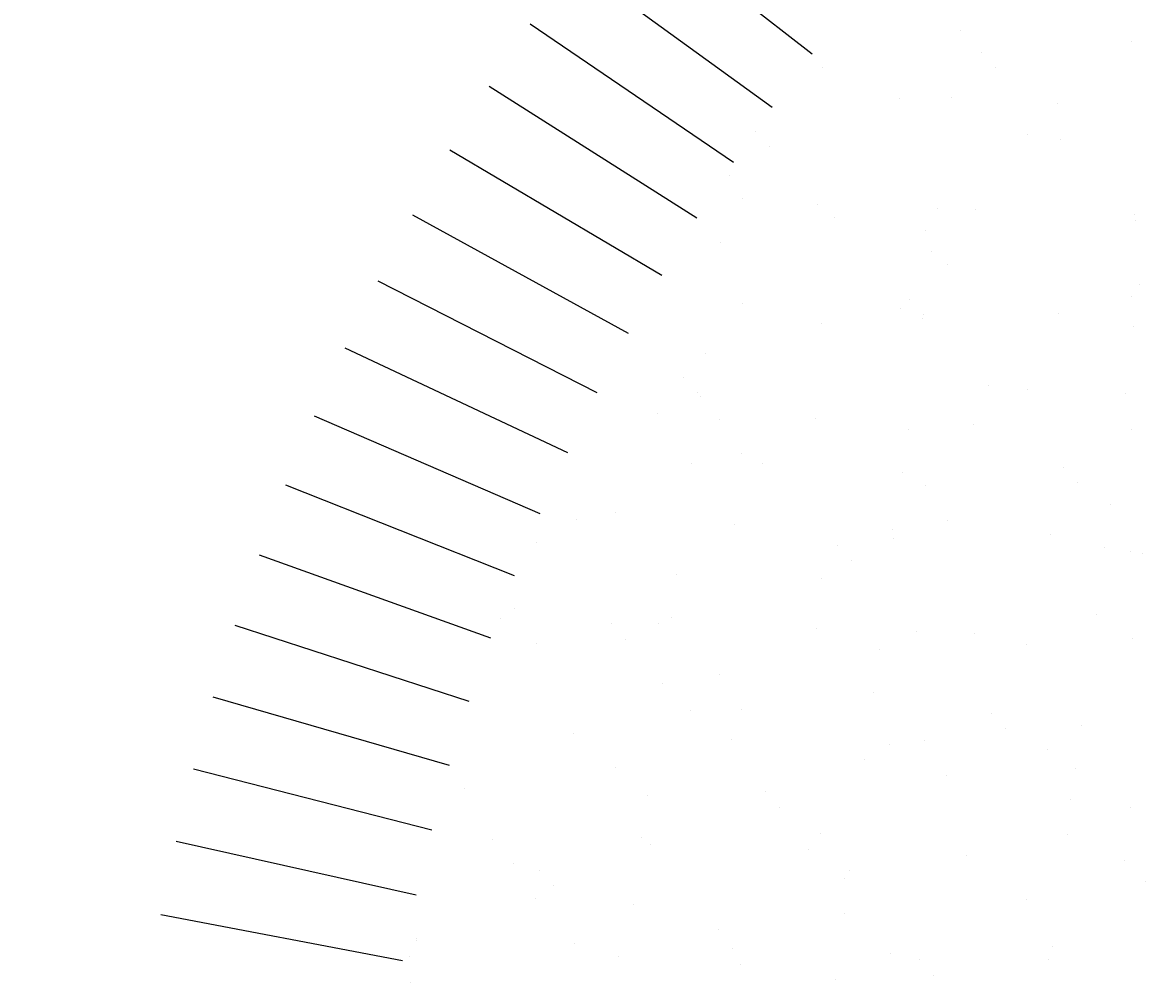
# Model space of a CAD drawing. Units: millimetres. Extents: x -857 to 54106, y -13666 to 13947.
# Tile 35 of 41: x 30856 to 31475, y 9986 to 10517. Entities that reach past the tile are written whole.
import ezdxf

# ---------------------------------------------------------------- set-up
doc = ezdxf.new("R2010")
doc.units = ezdxf.units.MM
doc.layers.add('A-ANNO-DIMS', color=2, linetype='Continuous', lineweight=18)
doc.layers.add('A-FURN', color=21, linetype='Continuous', lineweight=18)
doc.layers.add('A-HT', color=15, linetype='Continuous')
doc.styles.get("Standard").update_dxf_attribs({"font": 'arial.ttf'})
doc.dimstyles.new('ISO-25', dxfattribs={"dimtxt": 2.5, "dimasz": 2.5, "dimexe": 1.25, "dimexo": 0.625, "dimtad": 1, "dimtxsty": 'Standard', "dimcen": 2.5, "dimadec": 0, "dimazin": 0, "dimtfac": 1, "dimtmove": 0, "dimatfit": 3, "dimfxl": 1, "dimarcsym": 0})

# ---------------------------------------------------------------- blocks, each defined once
blk = doc.blocks.new('*X18')
at = {"color": 0}
for p, q in [((1.75374, 2.82274), (1.75374, 2.82274)), ((1.76978, 2.82215), (1.76978, 2.82215)), ((1.74276, 2.81864), (1.74276, 2.81864)), ((1.74375, 2.81872), (1.74375, 2.81872)), ((1.65142, 2.78914), (1.65142, 2.78914)), ((1.54742, 2.7675), (1.54742, 2.7675)), ((1.68246, 2.77237), (1.68246, 2.77237)), ((1.69713, 2.75932), (1.69713, 2.75932)), ((1.54142, 2.75904), (1.54142, 2.75904)), ((1.56251, 2.74561), (1.56251, 2.74561)), ((1.71821, 2.74589), (1.71821, 2.74589)), ((1.50111, 2.74526), (1.50111, 2.74526)), ((1.70118, 2.74354), (1.70118, 2.74354)), ((1.7104, 2.73509), (1.7104, 2.73509)), ((1.48712, 2.72124), (1.48712, 2.72124)), ((1.618, 2.72291), (1.618, 2.72291)), ((1.74591, 2.72229), (1.74591, 2.72229)), ((1.55088, 2.69965), (1.55088, 2.69965)), ((1.48271, 2.69697), (1.48271, 2.69697)), ((1.56009, 2.69121), (1.56009, 2.69121)), ((1.63841, 2.69725), (1.63841, 2.69725)), ((1.7539, 2.69523), (1.7539, 2.69523)), ((1.72194, 2.68639), (1.72194, 2.68639)), ((1.65526, 2.67761), (1.65526, 2.67761)), ((1.68129, 2.68104), (1.68129, 2.68104)), ((1.42266, 2.67178), (1.42266, 2.67178)), ((1.55057, 2.67116), (1.55057, 2.67116)), ((1.68561, 2.67603), (1.68561, 2.67603)), ((1.58735, 2.66867), (1.58735, 2.66867)), ((1.52067, 2.65989), (1.52067, 2.65989)), ((1.5467, 2.66332), (1.5467, 2.66332)), ((1.40057, 2.65577), (1.40057, 2.65577)), ((1.45276, 2.65095), (1.45276, 2.65095)), ((1.60359, 2.65135), (1.60359, 2.65135)), ((1.40979, 2.64732), (1.40979, 2.64732)), ((1.41211, 2.6456), (1.41211, 2.6456)), ((1.38609, 2.64217), (1.38609, 2.64217)), ((1.31817, 2.63323), (1.31817, 2.63323)), ((1.4261, 2.63355), (1.4261, 2.63355)), ((1.5818, 2.63383), (1.5818, 2.63383)), ((1.73751, 2.63412), (1.73751, 2.63412)), ((1.27752, 2.62788), (1.27752, 2.62788)), ((1.49027, 2.6249), (1.49027, 2.6249)), ((1.62115, 2.62657), (1.62115, 2.62657)), ((1.74906, 2.62595), (1.74906, 2.62595)), ((1.29147, 2.61984), (1.29147, 2.61984)), ((1.35523, 2.62003), (1.35523, 2.62003)), ((1.44718, 2.62012), (1.44718, 2.62012)), ((1.60289, 2.6204), (1.60289, 2.6204)), ((1.7586, 2.62069), (1.7586, 2.62069)), ((1.25027, 2.61189), (1.25027, 2.61189)), ((1.25948, 2.60344), (1.25948, 2.60344)), ((1.45329, 2.60747), (1.45329, 2.60747)), ((1.65336, 2.60575), (1.65336, 2.60575)), ((1.66258, 2.5973), (1.66258, 2.5973)), ((1.42581, 2.57544), (1.42581, 2.57544)), ((1.55372, 2.57482), (1.55372, 2.57482)), ((1.68876, 2.57969), (1.68876, 2.57969)), ((1.21167, 2.5712), (1.21167, 2.5712)), ((1.29493, 2.57377), (1.29493, 2.57377)), ((1.36738, 2.57148), (1.36738, 2.57148)), ((1.52309, 2.57176), (1.52309, 2.57176)), ((1.67879, 2.57205), (1.67879, 2.57205)), ((1.30298, 2.56358), (1.30298, 2.56358)), ((1.50305, 2.56186), (1.50305, 2.56186)), ((1.76804, 2.563), (1.76804, 2.563)), ((1.70136, 2.55422), (1.70136, 2.55422)), ((1.70607, 2.55744), (1.70607, 2.55744)), ((1.72739, 2.55765), (1.72739, 2.55765)), ((1.51227, 2.55342), (1.51227, 2.55342)), ((1.63345, 2.54528), (1.63345, 2.54528)), ((1.56677, 2.53651), (1.56677, 2.53651)), ((1.5928, 2.53993), (1.5928, 2.53993)), ((1.49342, 2.52856), (1.49342, 2.52856)), ((1.49886, 2.52756), (1.49886, 2.52756)), ((1.6243, 2.53023), (1.6243, 2.53023)), ((1.75221, 2.52961), (1.75221, 2.52961)), ((1.23047, 2.5243), (1.23047, 2.5243)), ((1.35838, 2.52369), (1.35838, 2.52369)), ((1.45821, 2.52221), (1.45821, 2.52221)), ((1.35275, 2.51798), (1.35275, 2.51798)), ((1.43218, 2.51879), (1.43218, 2.51879)), ((1.55577, 2.51356), (1.55577, 2.51356)), ((1.31077, 2.50806), (1.31077, 2.50806)), ((1.36196, 2.50953), (1.36196, 2.50953)), ((1.36427, 2.50985), (1.36427, 2.50985)), ((1.46648, 2.50835), (1.46648, 2.50835)), ((1.62219, 2.50863), (1.62219, 2.50863)), ((1.75584, 2.51184), (1.75584, 2.51184)), ((1.2976, 2.50107), (1.2976, 2.50107)), ((1.32362, 2.50449), (1.32362, 2.50449)), ((1.76506, 2.50339), (1.76506, 2.50339)), ((1.33186, 2.49463), (1.33186, 2.49463)), ((1.48756, 2.49491), (1.48756, 2.49491)), ((1.64327, 2.4952), (1.64327, 2.4952)), ((1.18903, 2.48677), (1.18903, 2.48677)), ((1.22968, 2.49213), (1.22968, 2.49213)), ((1.42896, 2.47909), (1.42896, 2.47909)), ((1.69191, 2.48335), (1.69191, 2.48335)), ((1.20244, 2.4741), (1.20244, 2.4741)), ((1.29808, 2.47743), (1.29808, 2.47743)), ((1.55687, 2.47848), (1.55687, 2.47848)), ((1.21166, 2.46565), (1.21166, 2.46565)), ((1.40546, 2.46967), (1.40546, 2.46967)), ((1.60553, 2.46796), (1.60553, 2.46796)), ((1.61475, 2.45951), (1.61475, 2.45951)), ((1.25205, 2.44599), (1.25205, 2.44599)), ((1.40776, 2.44627), (1.40776, 2.44627)), ((1.56347, 2.44656), (1.56347, 2.44656)), ((1.71918, 2.44684), (1.71918, 2.44684)), ((1.49657, 2.43222), (1.49657, 2.43222)), ((1.62745, 2.43388), (1.62745, 2.43388)), ((1.74746, 2.43084), (1.74746, 2.43084)), ((1.75536, 2.43327), (1.75536, 2.43327)), ((1.23362, 2.42796), (1.23362, 2.42796)), ((1.25516, 2.42579), (1.25516, 2.42579)), ((1.36153, 2.42735), (1.36153, 2.42735)), ((1.45523, 2.42407), (1.45523, 2.42407)), ((1.65825, 2.41965), (1.65825, 2.41965)), ((1.67955, 2.42189), (1.67955, 2.42189)), ((1.46444, 2.41563), (1.46444, 2.41563)), ((1.61287, 2.41312), (1.61287, 2.41312)), ((1.6389, 2.41654), (1.6389, 2.41654)), ((1.54496, 2.40418), (1.54496, 2.40418)), ((1.50431, 2.39882), (1.50431, 2.39882)), ((1.47828, 2.3954), (1.47828, 2.3954)), ((1.35115, 2.38286), (1.35115, 2.38286)), ((1.41037, 2.38646), (1.41037, 2.38646)), ((1.43211, 2.38275), (1.43211, 2.38275)), ((1.50686, 2.38314), (1.50686, 2.38314)), ((1.66257, 2.38342), (1.66257, 2.38342)), ((1.69506, 2.38701), (1.69506, 2.38701)), ((1.19545, 2.38258), (1.19545, 2.38258)), ((1.30123, 2.38108), (1.30123, 2.38108)), ((1.30492, 2.38019), (1.30492, 2.38019)), ((1.3437, 2.37768), (1.3437, 2.37768)), ((1.36972, 2.38111), (1.36972, 2.38111)), ((1.56002, 2.38214), (1.56002, 2.38214)), ((1.50794, 2.37577), (1.50794, 2.37577)), ((1.70802, 2.37405), (1.70802, 2.37405))]:
    blk.add_line(p, q, dxfattribs=at)
blk = doc.blocks.new('A$C6796526C')
at = {"layer": 'A-HT'}
for p, q in [((0.65322, 0.4228), (0.56128, 0.30428)), ((0.68588, 0.39828), (0.59771, 0.27693)), ((0.71929, 0.3748), (0.63498, 0.25073)), ((0.75343, 0.35237), (0.67305, 0.22572)), ((0.78825, 0.33104), (0.71189, 0.20192)), ((0.82372, 0.3108), (0.75146, 0.17936)), ((0.85981, 0.29169), (0.79171, 0.15804)), ((0.89649, 0.27372), (0.83262, 0.138)), ((0.93371, 0.25692), (0.87414, 0.11926)), ((0.97144, 0.24129), (0.91622, 0.10182)), ((1.00964, 0.22686), (0.95883, 0.08572)), ((1.04828, 0.21363), (1.00193, 0.07097)), ((1.08731, 0.20162), (1.04546, 0.05757)), ((1.1267, 0.19084), (1.0894, 0.04555)), ((1.16641, 0.18131), (1.13369, 0.03492)), ((1.2064, 0.17303), (1.1783, 0.02568))]:
    blk.add_line(p, q, dxfattribs=at)
at = {"layer": 'A-HT', "extrusion": (0, 0, -1), "zscale": -1, "rotation": 180}
blk.add_blockref('*X18', (0.55, 3), dxfattribs=at)
blk = doc.blocks.new('*D48')
at = {"layer": 'A-ANNO-DIMS', "color": 0, "lineweight": -2, "transparency": 16777216}
for p, q in [((30908.63, 11089.46), (30501.38, 11089.46)), ((30502.63, 11086.96), (30502.63, 8471.5)), ((30908.63, 8469), (30501.38, 8469))]:
    blk.add_line(p, q, dxfattribs=at)
at = {"layer": 'A-ANNO-DIMS', "color": 0, "transparency": 16777216}
for points in [[(30502.21, 11086.96), (30503.05, 11086.96), (30502.63, 11089.46)], [(30502.21, 8471.5), (30503.05, 8471.5), (30502.63, 8469)]]:
    blk.add_solid(points, dxfattribs=at)
at = {"layer": 'Defpoints', "color": 0, "transparency": 16777216}
for p in [(30909.25, 11089.46), (30502.63, 8469), (30909.25, 8469)]:
    blk.add_point(p, dxfattribs=at)
at = {"layer": 'A-ANNO-DIMS', "color": 0, "transparency": 16777216, "insert": (30500.73, 9779.23), "char_height": 2.5, "attachment_point": 5, "rotation": 90}
blk.add_mtext('2620 TYP.', dxfattribs=at)

msp = doc.modelspace()

# ---------------------------------------------------------------- block references
at = {"layer": 'A-FURN', "xscale": 903.6084929786902, "yscale": 903.6084929786902, "zscale": 903.6084929786902, "rotation": 269.9999999999988}
msp.add_blockref('A$C6796526C', (30909.253, 11089.463), dxfattribs=at)

# ---------------------------------------------------------------- dimensions: what is measured, and where the dimension line sits
at = {"layer": 'A-ANNO-DIMS'}
dim = msp.add_linear_dim(base=(30502.63, 8468.999), p1=(30909.254, 11089.463), p2=(30909.254, 8468.999), angle=270, text='<> TYP.', dimstyle='ISO-25', override={"dimdec": 0, "dimrnd": 0, "dimzin": 0, "dimlunit": 2}, dxfattribs=at)
dim.commit()
dim.dimension.update_dxf_attribs({"geometry": '*D48', "text_midpoint": (30500.728, 9779.231)})

doc.saveas('drawing.dxf')
